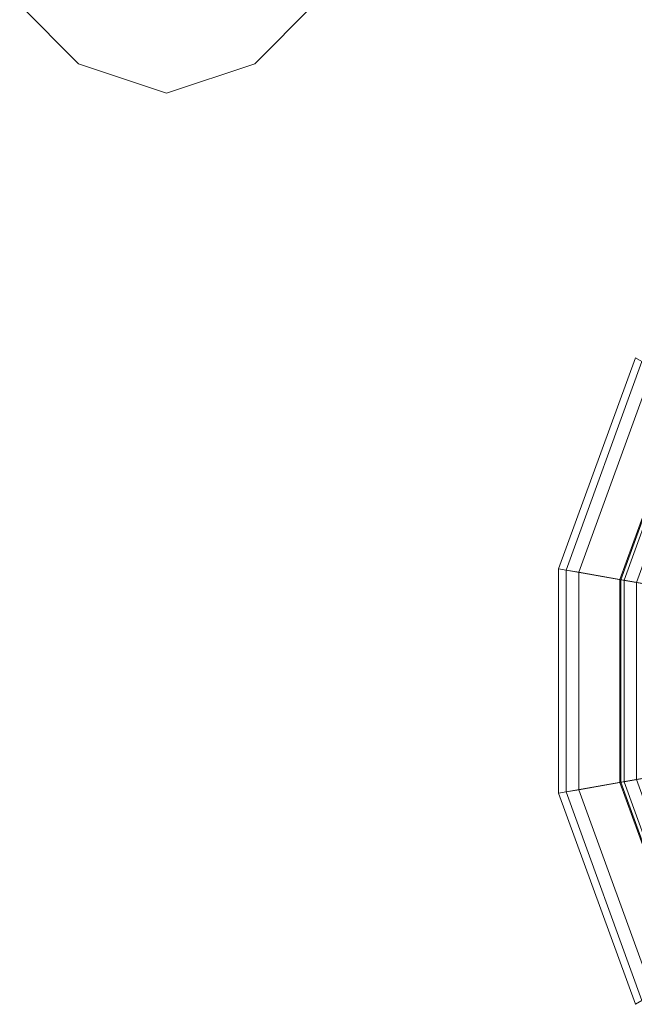
# Model space of a CAD drawing. Units: inches. Extents: x 375 to 1122, y 27 to 1069.
# Tile 47 of 155: x 719.619 to 720.906, y 309.788 to 311.85. Entities that reach past the tile are written whole.
import ezdxf

# ---------------------------------------------------------------- set-up
doc = ezdxf.new("R2010")
doc.units = ezdxf.units.IN
doc.layers.add('Furniture', color=30, linetype='Continuous', lineweight=18)

# ---------------------------------------------------------------- blocks, each defined once
blk = doc.blocks.new('A$C403C54AD')
for points in [[(0.878804, 0.899009, -0.042784), (0.895735, 0.928335, -0.039705), (0.895735, 0.928335, -0.039705), (0.889855, 0.894987, -0.042784)], [(0.889855, 0.894987, -0.042784), (0.895735, 0.928335, -0.039705), (0.895735, 0.928335, -0.039705), (0.901615, 0.894987, -0.042784)], [(0.901615, 0.894987, -0.042784), (0.895735, 0.928335, -0.039705), (0.895735, 0.928335, -0.039705), (0.912666, 0.899009, -0.042784)], [(0.888627, 0.916025, -0.036278), (0.880436, 0.901837, -0.039553), (0.890422, 0.898203, -0.039553), (0.893266, 0.914336, -0.036278)], [(0.898203, 0.914336, -0.036278), (0.901048, 0.898203, -0.039553), (0.911033, 0.901837, -0.039553), (0.902842, 0.916025, -0.036278)], [(0.893266, 0.914336, -0.036278), (0.890422, 0.898203, -0.039553), (0.901048, 0.898203, -0.039553), (0.898203, 0.914336, -0.036278)], [(0.882955, 0.906199, 0.129606), (0.880457, 0.901872, 0.1202), (0.890429, 0.898243, 0.1202), (0.891296, 0.903163, 0.129606)], [(0.900173, 0.903163, 0.129606), (0.901041, 0.898243, 0.1202), (0.911013, 0.901872, 0.1202), (0.908514, 0.906199, 0.129606)], [(0.87934, 0.899939, 0.078734), (0.882023, 0.904585, 0.060725), (0.890973, 0.901327, 0.060725), (0.890041, 0.896044, 0.078734)], [(0.880545, 0.902026, 0.106759), (0.88195, 0.904459, 0.119395), (0.890947, 0.901184, 0.119395), (0.890459, 0.898417, 0.106759)], [(0.901428, 0.896044, 0.078734), (0.900497, 0.901327, 0.060725), (0.909447, 0.904585, 0.060725), (0.912129, 0.899939, 0.078734)], [(0.90101, 0.898417, 0.106759), (0.900522, 0.901184, 0.119395), (0.909519, 0.904459, 0.119395), (0.910924, 0.902026, 0.106759)], [(0.891296, 0.903163, 0.129606), (0.890429, 0.898243, 0.1202), (0.901041, 0.898243, 0.1202), (0.900173, 0.903163, 0.129606)], [(0.880874, 0.902596, 0.079219), (0.880545, 0.902026, 0.106759), (0.890459, 0.898417, 0.106759), (0.890574, 0.899065, 0.079219)], [(0.900896, 0.899065, 0.079219), (0.90101, 0.898417, 0.106759), (0.910924, 0.902026, 0.106759), (0.910595, 0.902596, 0.079219)], [(0.880436, 0.901837, -0.039553), (0.878804, 0.899009, -0.042784), (0.889855, 0.894987, -0.042784), (0.890422, 0.898203, -0.039553)], [(0.880457, 0.901872, 0.1202), (0.879003, 0.899355, 0.106976), (0.889924, 0.89538, 0.106976), (0.890429, 0.898243, 0.1202)], [(0.901041, 0.898243, 0.1202), (0.901545, 0.89538, 0.106976), (0.912466, 0.899355, 0.106976), (0.911013, 0.901872, 0.1202)], [(0.901048, 0.898203, -0.039553), (0.901615, 0.894987, -0.042784), (0.912666, 0.899009, -0.042784), (0.911033, 0.901837, -0.039553)], [(0.890041, 0.896044, 0.078734), (0.890973, 0.901327, 0.060725), (0.900497, 0.901327, 0.060725), (0.901428, 0.896044, 0.078734)], [(0.890459, 0.898417, 0.106759), (0.890947, 0.901184, 0.119395), (0.900522, 0.901184, 0.119395), (0.90101, 0.898417, 0.106759)], [(0.879003, 0.899355, 0.106976), (0.87934, 0.899939, 0.078734), (0.890041, 0.896044, 0.078734), (0.889924, 0.89538, 0.106976)], [(0.901545, 0.89538, 0.106976), (0.901428, 0.896044, 0.078734), (0.912129, 0.899939, 0.078734), (0.912466, 0.899355, 0.106976)], [(0.890574, 0.899065, 0.079219), (0.890459, 0.898417, 0.106759), (0.90101, 0.898417, 0.106759), (0.900896, 0.899065, 0.079219)], [(0.890429, 0.898243, 0.1202), (0.889924, 0.89538, 0.106976), (0.901545, 0.89538, 0.106976), (0.901041, 0.898243, 0.1202)], [(0.890422, 0.898203, -0.039553), (0.889855, 0.894987, -0.042784), (0.901615, 0.894987, -0.042784), (0.901048, 0.898203, -0.039553)], [(0.889924, 0.89538, 0.106976), (0.890041, 0.896044, 0.078734), (0.901428, 0.896044, 0.078734), (0.901545, 0.89538, 0.106976)]]:
    blk.add_3dface(points)
for points, invisible_edges in [([(0.863412, 0.869845, -0.035857), (0.863412, 0.87908, -0.035857), (0.860333, 0.882159, -0.035857), (0.860333, 0.866767, -0.035857)], 5), ([(0.863412, 0.869845, -0.037397), (0.863412, 0.87908, -0.037397), (0.860333, 0.882159, -0.037397), (0.860333, 0.866767, -0.037397)], 5), ([(0.863412, 0.87908, -0.037397), (0.863412, 0.87908, -0.035857), (0.860333, 0.882159, -0.035857), (0.860333, 0.882159, -0.037397)], 5), ([(0.864951, 0.874463, -0.035857), (0.864951, 0.874463, -0.035857), (0.863412, 0.869845, -0.035857), (0.863412, 0.87908, -0.035857)], 4), ([(0.864951, 0.874463, -0.037397), (0.864951, 0.874463, -0.037397), (0.863412, 0.869845, -0.037397), (0.863412, 0.87908, -0.037397)], 4), ([(0.864951, 0.874463, -0.035857), (0.864951, 0.874463, -0.037397), (0.863412, 0.87908, -0.037397), (0.863412, 0.87908, -0.035857)], 4), ([(0.863412, 0.869845, -0.037397), (0.863412, 0.869845, -0.035857), (0.864951, 0.874463, -0.035857), (0.864951, 0.874463, -0.037397)], 1), ([(0.860333, 0.866767, -0.035857), (0.860333, 0.866767, -0.037397), (0.863412, 0.869845, -0.037397), (0.863412, 0.869845, -0.035857)], 5)]:
    blk.add_3dface(points, dxfattribs=dict(invisible_edges=invisible_edges))

msp = doc.modelspace()

# ---------------------------------------------------------------- block references
at = {"layer": 'Furniture', "xscale": 39.9918517141215, "yscale": 39.9918517141215, "zscale": 39.9918517141215, "rotation": 270}
msp.add_blockref('A$C403C54AD', (684.9549, 346.2875, 0.024), dxfattribs=at)

doc.saveas('drawing.dxf')
